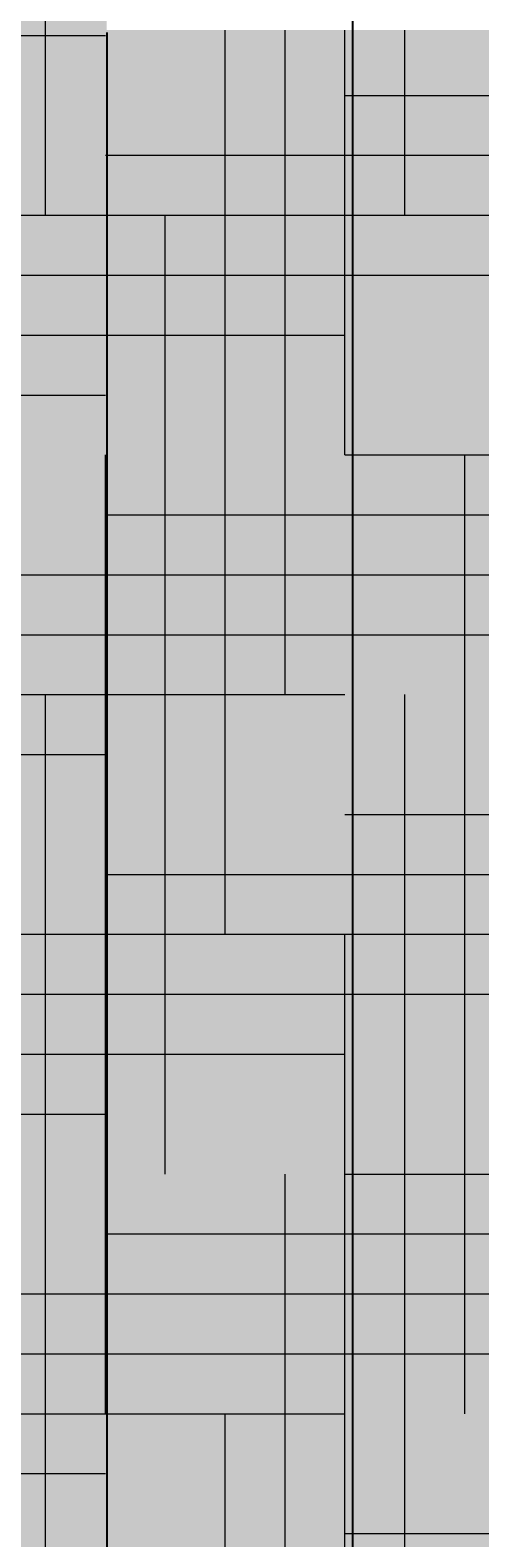
# Model space of a CAD drawing. Units: feet. Extents: x 2695 to 2912, y 795 to 1139.
# Tile 7 of 83: x 2722 to 2734, y 835 to 875. Entities that reach past the tile are written whole.
import ezdxf

# ---------------------------------------------------------------- set-up
doc = ezdxf.new("R2010")
doc.units = ezdxf.units.FT
doc.layers.add('A-ANNO-DIMS', color=2, linetype='Continuous', lineweight=18)
doc.layers.add('A-ELEV-PATT', color=252, linetype='Continuous', lineweight=13)
doc.styles.get("Standard").update_dxf_attribs({"font": 'arial.ttf'})
doc.dimstyles.get("Standard").update_dxf_attribs({"dimtxt": 0.18, "dimasz": 0.18, "dimexe": 0.18, "dimexo": 0.0625, "dimgap": 0.09, "dimtad": 0, "dimtih": 1, "dimtoh": 1, "dimdec": 1, "dimzin": 0, "dimdsep": 46, "dimlunit": 3, "dimtxsty": 'Standard', "dimcen": 0.09, "dimadec": 0, "dimazin": 0, "dimtfac": 1, "dimtdec": 1, "dimtofl": 0, "dimtmove": 0, "dimatfit": 3, "dimfxl": 1, "dimtolj": 1, "dimtzin": 0, "dimarcsym": 0})

# ---------------------------------------------------------------- blocks, each defined once
blk = doc.blocks.new('*D2')
at = {"layer": 'A-ANNO-DIMS', "color": 0, "lineweight": -2, "transparency": 16777216}
for p, q in [((2724.189, 874.795), (2724.189, 794.976)), ((2716.536, 810.868), (2716.536, 794.976)), ((2716.716, 795.156), (2719.97, 795.156)), ((2724.009, 795.156), (2720.756, 795.156))]:
    blk.add_line(p, q, dxfattribs=at)
at = {"layer": 'A-ANNO-DIMS', "color": 0, "transparency": 16777216}
for points in [[(2716.716, 795.186), (2716.716, 795.126), (2716.536, 795.156)], [(2724.009, 795.186), (2724.009, 795.126), (2724.189, 795.156)]]:
    blk.add_solid(points, dxfattribs=at)
at = {"layer": 'Defpoints', "color": 0, "transparency": 16777216}
for p in [(2724.189, 874.857), (2716.536, 810.931), (2724.189, 795.156)]:
    blk.add_point(p, dxfattribs=at)
at = {"layer": 'A-ANNO-DIMS', "color": 0, "transparency": 16777216, "insert": (2720.363, 795.156), "char_height": 0.18, "attachment_point": 5}
blk.add_mtext('\\A1;7.653', dxfattribs=at)
blk = doc.blocks.new('*D3')
at = {"layer": 'A-ANNO-DIMS', "color": 0, "lineweight": -2, "transparency": 16777216}
for p, q in [((2724.189, 874.795), (2724.189, 794.976)), ((2758.151, 874.795), (2758.151, 794.976)), ((2724.369, 795.156), (2740.777, 795.156)), ((2757.971, 795.156), (2741.564, 795.156))]:
    blk.add_line(p, q, dxfattribs=at)
at = {"layer": 'A-ANNO-DIMS', "color": 0, "transparency": 16777216}
for points in [[(2724.369, 795.186), (2724.369, 795.126), (2724.189, 795.156)], [(2757.971, 795.186), (2757.971, 795.126), (2758.151, 795.156)]]:
    blk.add_solid(points, dxfattribs=at)
at = {"layer": 'Defpoints', "color": 0, "transparency": 16777216}
for p in [(2724.189, 874.857), (2758.151, 874.857), (2758.151, 795.156)]:
    blk.add_point(p, dxfattribs=at)
at = {"layer": 'A-ANNO-DIMS', "color": 0, "transparency": 16777216, "insert": (2741.17, 795.156), "char_height": 0.18, "attachment_point": 5}
blk.add_mtext('\\A1;33.96', dxfattribs=at)
blk = doc.blocks.new('*D23')
at = {"layer": 'A-ANNO-DIMS', "color": 0, "lineweight": -2, "transparency": 16777216}
for p, q in [((2715.885, 936.868), (2715.885, 794.976)), ((2730.708, 936.868), (2730.708, 794.976)), ((2716.065, 795.156), (2722.842, 795.156)), ((2730.528, 795.156), (2723.752, 795.156))]:
    blk.add_line(p, q, dxfattribs=at)
at = {"layer": 'A-ANNO-DIMS', "color": 0, "transparency": 16777216}
for points in [[(2716.065, 795.186), (2716.065, 795.126), (2715.885, 795.156)], [(2730.528, 795.186), (2730.528, 795.126), (2730.708, 795.156)]]:
    blk.add_solid(points, dxfattribs=at)
at = {"layer": 'Defpoints', "color": 0, "transparency": 16777216}
for p in [(2715.885, 936.931), (2730.708, 936.931), (2730.708, 795.156)]:
    blk.add_point(p, dxfattribs=at)
at = {"layer": 'A-ANNO-DIMS', "color": 0, "transparency": 16777216, "insert": (2723.297, 795.156), "char_height": 0.18, "attachment_point": 5}
blk.add_mtext('\\A1;14.823', dxfattribs=at)
blk = doc.blocks.new('*D24')
at = {"layer": 'A-ANNO-DIMS', "color": 0, "lineweight": -2, "transparency": 16777216}
for p, q in [((2730.708, 936.868), (2730.708, 794.976)), ((2755.112, 936.868), (2755.112, 794.976)), ((2730.888, 795.156), (2742.446, 795.156)), ((2754.932, 795.156), (2743.375, 795.156))]:
    blk.add_line(p, q, dxfattribs=at)
at = {"layer": 'A-ANNO-DIMS', "color": 0, "transparency": 16777216}
for points in [[(2730.888, 795.186), (2730.888, 795.126), (2730.708, 795.156)], [(2754.932, 795.186), (2754.932, 795.126), (2755.112, 795.156)]]:
    blk.add_solid(points, dxfattribs=at)
at = {"layer": 'Defpoints', "color": 0, "transparency": 16777216}
for p in [(2730.708, 936.931), (2755.112, 936.931), (2755.112, 795.156)]:
    blk.add_point(p, dxfattribs=at)
at = {"layer": 'A-ANNO-DIMS', "color": 0, "transparency": 16777216, "insert": (2742.91, 795.156), "char_height": 0.18, "attachment_point": 5}
blk.add_mtext('\\A1;24.404', dxfattribs=at)

msp = doc.modelspace()

# ---------------------------------------------------------------- hatches: boundary and pattern name
at = {"layer": 'A-ELEV-PATT'}
h = msp.add_hatch(color=256, dxfattribs=at)
h.set_gradient(color1=(255, 255, 255))
h.paths.add_polyline_path([(2770.6361, 924.3105), (2716.5358, 924.3105), (2716.5358, 810.9306), (2770.6361, 810.9306)])
h.paths.add_polyline_path([(2758.1515, 902.577), (2758.1515, 874.8571), (2724.1893, 874.8571), (2724.1893, 902.577)], flags=16)
h.paths.add_polyline_path([(2756.1515, 900.577), (2756.1515, 876.8571), (2726.1893, 876.8571), (2726.1893, 900.577)], flags=0)
h.paths.add_polyline_path([(2740.7302, 900.577), (2741.6105, 900.577), (2741.6105, 876.8571), (2740.7302, 876.8571)], flags=0)
h = msp.add_hatch(dxfattribs=at)
h.set_pattern_fill('HOUND', color=256, style=0)
h.paths.add_polyline_path([(2770.6361, 924.3105), (2716.5358, 924.3105), (2716.5358, 810.9306), (2770.6361, 810.9306)])
h.paths.add_polyline_path([(2724.1893, 874.8571), (2724.1893, 902.577), (2758.1515, 902.577), (2758.1515, 874.8571)], flags=16)
h.paths.add_polyline_path([(2756.1515, 876.8571), (2726.1893, 876.8571), (2726.1893, 900.577), (2756.1515, 900.577)], flags=0)
h.paths.add_polyline_path([(2741.6105, 876.8571), (2740.7302, 876.8571), (2740.7302, 900.577), (2741.6105, 900.577)], flags=0)

# ---------------------------------------------------------------- dimensions: what is measured, and where the dimension line sits
at = {"layer": 'A-ANNO-DIMS'}
for base, p1, p2, override, picture, middle in [((2730.7081, 795.1556), (2715.8852, 936.9306), (2730.7081, 936.9306), {"dimdec": 3, "dimlfac": 1, "dimrnd": 0, "dimzin": 0, "dimdsep": 46, "dimlunit": 2}, '*D23', (2723.2967, 795.1556)), ((2755.1125, 795.1556), (2730.7081, 936.9306), (2755.1125, 936.9306), {"dimdec": 3, "dimlfac": 1, "dimrnd": 0, "dimzin": 0, "dimdsep": 46, "dimlunit": 2}, '*D24', (2742.9103, 795.1556)), ((2724.18927, 795.15559), (2716.53582, 810.93059), (2724.18927, 874.85709), {"dimdec": 3, "dimlfac": 1, "dimrnd": 0, "dimzin": 0, "dimdsep": 46, "dimlunit": 2}, '*D2', (2720.36254, 795.15559)), ((2758.1515, 795.1556), (2724.1893, 874.8571), (2758.1515, 874.8571), {"dimdec": 2, "dimlfac": 1, "dimrnd": 0, "dimzin": 0, "dimdsep": 46, "dimlunit": 2}, '*D3', (2741.1704, 795.1556))]:
    dim = msp.add_linear_dim(base=base, p1=p1, p2=p2, dimstyle='Standard', override=override, dxfattribs=at)
    dim.commit()
    dim.dimension.update_dxf_attribs({"geometry": picture, "text_midpoint": middle})

doc.saveas('drawing.dxf')
